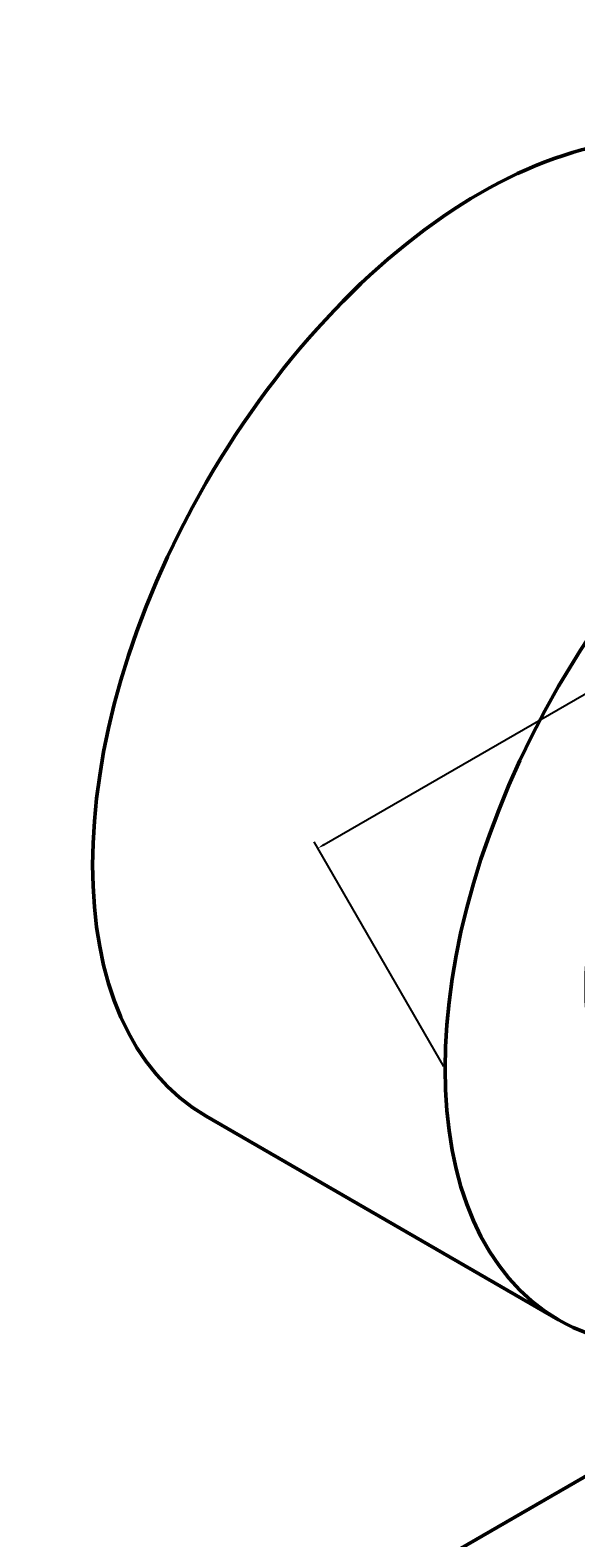
# Model space of a CAD drawing. Units: inches. Extents: x -23 to 69, y -27 to 96.
# Tile 6 of 10: x -2 to 11, y 35 to 72. Entities that reach past the tile are written whole.
import ezdxf

# ---------------------------------------------------------------- set-up
doc = ezdxf.new("R2010")
doc.units = ezdxf.units.IN
doc.header["$MEASUREMENT"] = 0
doc.layers.add('M-DIMS', color=2, linetype='Continuous', lineweight=18)
doc.layers.add('M-OUTL', color=7, linetype='Continuous', lineweight=50)
doc.styles.get("Standard").update_dxf_attribs({"font": 'arial.ttf'})
doc.dimstyles.get("Standard").update_dxf_attribs({"dimtxt": 0.18, "dimasz": 0.18, "dimexe": 0.18, "dimexo": 0.0625, "dimgap": 0.09, "dimtad": 0, "dimtih": 1, "dimtoh": 1, "dimdec": 4, "dimzin": 0, "dimdsep": 46, "dimtxsty": 'Standard', "dimcen": 0.09, "dimadec": 0, "dimazin": 0, "dimtfac": 1, "dimtdec": 4, "dimtofl": 0, "dimtmove": 0, "dimatfit": 3, "dimfxl": 1, "dimtolj": 1, "dimtzin": 0, "dimarcsym": 0})

# ---------------------------------------------------------------- blocks, each defined once
blk = doc.blocks.new('*D11')
at = {"layer": 'Defpoints', "color": 0, "transparency": 16777216}
for p in [(23.972, 63.031), (27.097, 57.619), (8.044, 46.619)]:
    blk.add_point(p, dxfattribs=at)
at = {"layer": 'M-DIMS', "color": 0, "lineweight": -2, "transparency": 16777216}
for p, q in [((23.816, 62.941), (14.761, 57.714)), ((27.065, 57.673), (23.882, 63.187)), ((5.075, 52.121), (14.129, 57.349)), ((8.013, 46.673), (4.829, 52.187))]:
    blk.add_line(p, q, dxfattribs=at)
at = {"layer": 'M-DIMS', "color": 0, "transparency": 16777216}
for points in [[(23.801, 62.967), (23.831, 62.915), (23.972, 63.031)], [(5.06, 52.147), (5.09, 52.095), (4.919, 52.031)]]:
    blk.add_solid(points, dxfattribs=at)
at = {"layer": 'M-DIMS', "color": 0, "transparency": 16777216, "insert": (14.445, 57.531), "char_height": 0.18, "attachment_point": 5}
blk.add_mtext('\\A1;%%c22', dxfattribs=at)
blk = doc.blocks.new('*D13')
at = {"layer": 'Defpoints', "color": 0, "transparency": 16777216}
for p in [(15.838, 89.119), (-22.888, -20.881), (36.623, -20.881)]:
    blk.add_point(p, dxfattribs=at)
at = {"layer": 'M-DIMS', "color": 0, "lineweight": -2, "transparency": 16777216}
for p, q in [((15.776, 89.119), (-23.068, 89.119)), ((-22.888, 88.939), (-22.888, 34.301)), ((-22.888, -20.701), (-22.888, 33.937)), ((36.56, -20.881), (-23.068, -20.881))]:
    blk.add_line(p, q, dxfattribs=at)
at = {"layer": 'M-DIMS', "color": 0, "transparency": 16777216}
for points in [[(-22.918, 88.939), (-22.858, 88.939), (-22.888, 89.119)], [(-22.918, -20.701), (-22.858, -20.701), (-22.888, -20.881)]]:
    blk.add_solid(points, dxfattribs=at)
at = {"layer": 'M-DIMS', "color": 0, "transparency": 16777216, "insert": (-22.888, 34.119), "char_height": 0.18, "attachment_point": 5}
blk.add_mtext('\\A1;110', dxfattribs=at)
blk = doc.blocks.new('*D16')
at = {"layer": 'Defpoints', "color": 0, "transparency": 16777216}
for p in [(17.57, 95.369), (-8.41, 69.119), (17.57, 52.119)]:
    blk.add_point(p, dxfattribs=at)
at = {"layer": 'M-DIMS', "color": 0, "lineweight": -2, "transparency": 16777216}
for p, q in [((-8.41, 69.181), (-8.41, 95.549)), ((17.57, 52.181), (17.57, 95.549)), ((-8.23, 95.369), (4.184, 95.369)), ((17.39, 95.369), (4.975, 95.369))]:
    blk.add_line(p, q, dxfattribs=at)
at = {"layer": 'M-DIMS', "color": 0, "transparency": 16777216}
for points in [[(-8.23, 95.399), (-8.23, 95.339), (-8.41, 95.369)], [(17.39, 95.399), (17.39, 95.339), (17.57, 95.369)]]:
    blk.add_solid(points, dxfattribs=at)
at = {"layer": 'M-DIMS', "color": 0, "transparency": 16777216, "insert": (4.58, 95.369), "char_height": 0.18, "attachment_point": 5}
blk.add_mtext('\\A1;25.98', dxfattribs=at)

msp = doc.modelspace()

# ---------------------------------------------------------------- linework, layer by layer
at = {"layer": 'M-OUTL'}
for p, q in [((34.4578, 49.8686), (-11.4416, 23.3686)), ((2.1739, 45.4514), (10.8342, 40.4514))]:
    msp.add_line(p, q, dxfattribs=at)
msp.add_ellipse((8.91, 57.1186), major_axis=(-6.7361, -11.6673), ratio=0.5773503, start_param=3.1415927, end_param=6.2831853, dxfattribs=at)
for major_axis in [(-6.7361, -11.6673), (-4.2866, -7.4246)]:
    msp.add_ellipse((17.5703, 52.1186), major_axis=major_axis, ratio=0.5773503, dxfattribs=at)

# ---------------------------------------------------------------- dimensions: what is measured, and where the dimension line sits
at = {"layer": 'M-DIMS'}
dim = msp.add_linear_dim(base=(17.5703, 95.3686), p1=(-8.4105, 69.1186), p2=(17.5703, 52.1186), dimstyle='Standard', override={"dimdec": 2, "dimlfac": 1, "dimrnd": 0, "dimzin": 0, "dimdsep": 46, "dimlunit": 2}, dxfattribs=at)
dim.commit()
dim.dimension.update_dxf_attribs({"geometry": '*D16', "text_midpoint": (4.5799, 95.3686)})
dim = msp.add_linear_dim(base=(-22.8877, -20.8814), p1=(15.8382, 89.1186), p2=(36.6228, -20.8814), angle=90, dimstyle='Standard', override={"dimdec": 0, "dimlfac": 1, "dimrnd": 0, "dimzin": 0, "dimdsep": 46, "dimlunit": 2}, dxfattribs=at)
dim.commit()
dim.dimension.update_dxf_attribs({"geometry": '*D13', "text_midpoint": (-22.8877, 34.1186)})
dim = msp.add_linear_dim(base=(23.9715, 63.0313), p1=(8.044, 46.6186), p2=(27.0965, 57.6186), angle=30, text='%%c<>', dimstyle='Standard', override={"dimdec": 0, "dimlfac": 1, "dimrnd": 0, "dimzin": 0, "dimdsep": 46, "dimlunit": 2}, dxfattribs=at)
dim.commit()
dim.dimension.update_dxf_attribs({"geometry": '*D11', "text_midpoint": (14.4453, 57.5313)})

doc.saveas('drawing.dxf')
